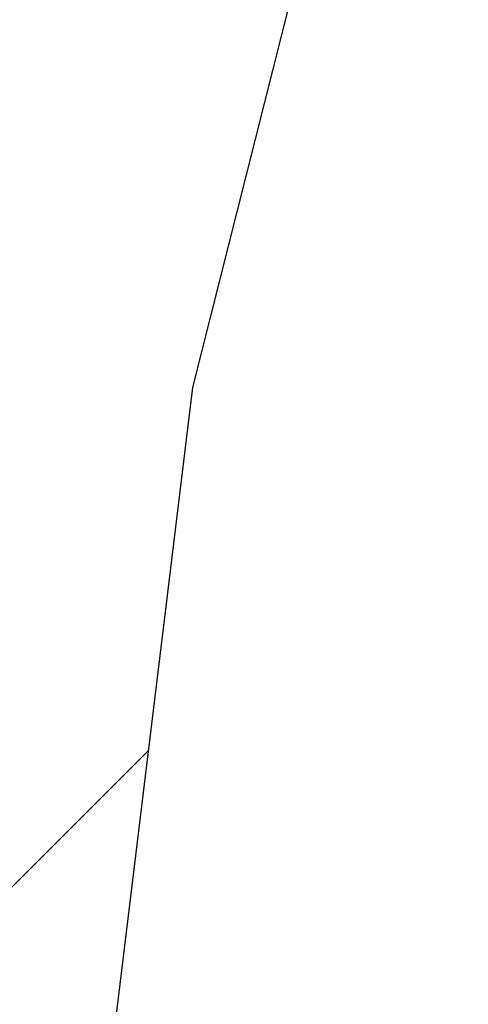
# Model space of a CAD drawing. Units: inches. Extents: x 3590 to 5167, y 65 to 1917.
# Tile 79 of 100: x 5049.155 to 5050.01, y 1787.154 to 1789.032. Entities that reach past the tile are written whole.
import ezdxf

# ---------------------------------------------------------------- set-up
doc = ezdxf.new("R2010")
doc.units = ezdxf.units.IN
for name, color, linetype, lineweight in [('A-ANNO-DIMS', 2, 'Continuous', 18), ('A-FLOR-PATT', 8, 'Continuous', 13), ('L-PLNT', 94, 'Continuous', 18)]:
    doc.layers.add(name, color=color, linetype=linetype, lineweight=lineweight)
doc.layers.add('DIENHOA', color=3, linetype='Continuous')
doc.styles.get("Standard").update_dxf_attribs({"font": 'arial.ttf'})
doc.dimstyles.new('ISO-25', dxfattribs={"dimtxt": 9, "dimasz": 2.5, "dimexe": 1.25, "dimexo": 0.625, "dimtad": 1, "dimdec": 1, "dimlunit": 3, "dimtxsty": 'Standard', "dimcen": 2.5, "dimadec": 0, "dimazin": 0, "dimtfac": 1, "dimtdec": 1, "dimtmove": 0, "dimatfit": 3, "dimfxl": 1, "dimarcsym": 0})

# ---------------------------------------------------------------- blocks, each defined once
blk = doc.blocks.new('Cay03_mb')
at = {"layer": 'DIENHOA'}
blk.add_lwpolyline([(-16.392, -26.735), (-38.342, 79.959), (-48.875, 178.33), (-48.703, 268.997), (-38.535, 352.583), (-19.079, 429.708), (8.954, 500.992), (44.855, 567.058), (87.915, 628.525)], dxfattribs=at)
blk = doc.blocks.new('*D322')
at = {"layer": 'A-ANNO-DIMS', "color": 0, "lineweight": -2, "transparency": 16777216}
for p, q in [((5035.7437, 1766.1842), (5035.7437, 1761.199)), ((5064.812, 1766.1842), (5064.812, 1761.199)), ((5038.2437, 1762.449), (5062.312, 1762.449)), ((5064.812, 1762.449), (5166.9911, 1762.449))]:
    blk.add_line(p, q, dxfattribs=at)
at = {"layer": 'A-ANNO-DIMS', "color": 0, "transparency": 16777216}
for points in [[(5038.2437, 1762.8657), (5038.2437, 1762.0323), (5035.7437, 1762.449)], [(5062.312, 1762.8657), (5062.312, 1762.0323), (5064.812, 1762.449)]]:
    blk.add_solid(points, dxfattribs=at)
at = {"layer": 'Defpoints', "color": 0, "transparency": 16777216}
for p in [(5035.7437, 1766.8092), (5064.812, 1766.8092), (5064.812, 1762.449)]:
    blk.add_point(p, dxfattribs=at)
at = {"layer": 'A-ANNO-DIMS', "color": 0, "transparency": 16777216, "insert": (5117.1516, 1767.6692), "char_height": 9, "attachment_point": 5}
blk.add_mtext('PLANT 2\'-5" TYP.', dxfattribs=at)

msp = doc.modelspace()

# ---------------------------------------------------------------- hatches: boundary and pattern name
at = {"layer": 'A-FLOR-PATT', "transparency": 33554687}
h = msp.add_hatch(dxfattribs=at)
h.set_pattern_fill('AR-HBONE', color=256, scale=0.2)
h.set_pattern_definition([(45, (-588.972, 0), (0, 28.73682), [60.96, -20.32]), (135, (-574.604, 14.368), (3e-15, 28.73682), [60.96, -20.32])])
h.paths.add_polyline_path([(5071.274, 1796.999), (4933.274, 1796.999), (4933.274, 1753.999), (4962.774, 1753.999, -0.414214), (4928.774, 1719.999), (4933.274, 1718.999), (4933.274, 1334.999), (5071.274, 1334.999)])
h.paths.add_polyline_path([(4951.78, 1521.0767), (4951.7151, 1521.0404), (4951.5634, 1520.8953)], flags=16)
h.paths.add_polyline_path([(4952.267, 1521.3764), (4952.1977, 1521.3711), (4952.1982, 1521.3556)], flags=0)
h.paths.add_polyline_path([(4967.0508, 1529.7283), (4965.2312, 1528.6944), (4963.4111, 1527.714), (4961.7565, 1526.8508), (4963.5889, 1527.4494), (4964.0356, 1527.478), (4962.9755, 1527.249), (4961.7602, 1526.852), (4959.7922, 1525.8341), (4958.005, 1524.8948), (4956.2403, 1523.9296), (4954.5039, 1522.9185), (4954.1294, 1522.6816), (4953.3605, 1521.9969), (4953.3656, 1521.9975), (4953.605, 1522.0637), (4955.1061, 1522.7608), (4956.9211, 1523.4341), (4958.6778, 1523.9151), (4960.3583, 1524.2004), (4961.9446, 1524.2861), (4964.1714, 1524.1085), (4965.9575, 1523.309), (4963.8627, 1522.9756), (4965.1874, 1522.499), (4963.3661, 1522.4971), (4961.5453, 1522.4868), (4959.7636, 1522.4608), (4958.3041, 1522.4188), (4957.9736, 1522.3883), (4956.3069, 1522.2324), (4954.7182, 1522.0714), (4953.2508, 1521.8992), (4953.5251, 1521.6228), (4954.3309, 1521.3788), (4956.2426, 1521.2299), (4958.0391, 1520.9295), (4959.6842, 1520.4834), (4961.1601, 1519.8957), (4963.107, 1518.8002), (4964.3929, 1517.3252), (4962.9731, 1517.726), (4964.5584, 1516.6606), (4965.4066, 1515.7078), (4963.5073, 1516.3218), (4961.68, 1517.0051), (4959.9348, 1517.7449), (4958.2821, 1518.5283), (4956.7322, 1519.3426), (4955.2953, 1520.1748), (4954.6715, 1520.5724), (4954.5128, 1520.6271), (4955.6585, 1519.3184), (4956.7026, 1517.9823), (4957.644, 1516.6466), (4958.4855, 1515.3344), (4959.55, 1513.524), (4960.4377, 1511.7694), (4958.8411, 1513.6196), (4957.4517, 1515.3249), (4955.8186, 1517.4586), (4956.6654, 1515.4476), (4957.1111, 1513.9229), (4957.4468, 1511.7143), (4957.0764, 1509.7929), (4956.5376, 1511.1103), (4955.9923, 1512.5689), (4955.4445, 1514.1251), (4954.8979, 1515.7352), (4954.3565, 1517.3555), (4953.8241, 1518.9425), (4953.3046, 1520.4525), (4953.0645, 1521.1156), (4952.9714, 1521.1461), (4952.9493, 1521.0865), (4952.7298, 1520.199), (4953.3698, 1518.0236), (4953.7571, 1516.3728), (4954.0512, 1514.7654), (4954.2645, 1513.2212), (4954.4712, 1511.1312), (4954.4971, 1510.4017), (4954.409, 1511.7601), (4954.2645, 1513.2212), (4954.0512, 1514.7654), (4953.7571, 1516.3728), (4953.3698, 1518.0236), (4952.8772, 1519.6981), (4952.7161, 1520.1412), (4952.533, 1519.0587), (4952.3743, 1517.7888), (4952.2192, 1516.3117), (4952.046, 1514.5999), (4951.8325, 1512.626), (4951.557, 1510.3626), (4951.2033, 1512.1682), (4950.8517, 1514.3393), (4950.9853, 1516.3759), (4951.6596, 1518.2862), (4952.5926, 1520.4808), (4952.3566, 1521.1299), (4951.855, 1520.3275), (4950.839, 1518.9083), (4949.7767, 1517.5866), (4948.9155, 1516.6173), (4948.111, 1515.2561), (4947.0891, 1513.5539), (4945.8894, 1511.6149), (4946.3259, 1513.4023), (4946.5624, 1514.2491), (4945.5277, 1513.3267), (4944.5811, 1512.5313), (4946.0177, 1514.5082), (4947.2044, 1516.0476), (4947.8933, 1517.3133), (4949.3069, 1518.7645), (4950.4142, 1519.7672), (4950.4513, 1519.8063), (4952.267, 1521.3764), (4951.6446, 1521.4932), (4950.4037, 1521.1795), (4948.0445, 1520.3587), (4946.1186, 1519.452), (4944.5718, 1518.4748), (4943.3496, 1517.4427), (4941.997, 1515.9197), (4941.6615, 1515.2748), (4942.8133, 1516.9897), (4944.5718, 1518.4748), (4946.1186, 1519.452), (4948.0445, 1520.3587), (4950.4037, 1521.1795), (4951.6446, 1521.4932), (4949.6468, 1521.8678), (4948.5998, 1521.7563), (4947.1263, 1521.5699), (4945.4202, 1521.3476), (4943.4497, 1521.1046), (4941.1832, 1520.856), (4942.8603, 1521.6126), (4943.8731, 1522.0301), (4942.9522, 1521.9093), (4941.4097, 1521.4851), (4939.5429, 1520.6702), (4938.9677, 1520.2255), (4940.7328, 1521.299), (4942.9522, 1521.9093), (4943.7018, 1522.0077), (4945.8942, 1522.7), (4947.5649, 1522.714), (4948.9209, 1522.5657), (4951.1314, 1522.1827), (4950.9706, 1522.2969), (4948.1292, 1523.0056), (4946.035, 1523.7067), (4944.2323, 1524.5214), (4942.7069, 1525.4611), (4941.4442, 1526.5371), (4940.4297, 1527.7606), (4939.6489, 1529.1431), (4941.4209, 1528.1223), (4943.1474, 1527.1325), (4944.8409, 1526.1746), (4946.5139, 1525.2496), (4948.1789, 1524.3586), (4948.3646, 1524.2634), (4946.4753, 1526.0446), (4945.1808, 1527.5404), (4944.1904, 1529.0334), (4943.4956, 1530.5398), (4943.2781, 1531.3597), (4942.4985, 1531.919), (4943.1135, 1531.7625), (4942.9593, 1533.6586), (4944.1395, 1531.9886), (4944.6117, 1531.3234), (4946.2016, 1530.4634), (4947.4857, 1529.5093), (4948.7903, 1528.2265), (4950.3675, 1526.2375), (4949.4855, 1528.1555), (4948.8513, 1530.1225), (4948.4905, 1532.0413), (4948.3811, 1533.9182), (4948.5006, 1535.7599), (4948.827, 1537.5728), (4949.418, 1535.5653), (4949.9568, 1533.5693), (4950.4641, 1531.5861), (4950.9606, 1529.6167), (4951.3911, 1527.9545), (4951.7235, 1530.6869), (4952.2011, 1532.5799), (4952.8891, 1534.3296), (4953.7703, 1535.9512), (4954.8273, 1537.46), (4954.5214, 1535.3897), (4954.2731, 1533.9368), (4955.58, 1535.6627), (4956.7476, 1536.7386), (4956.1585, 1534.7803), (4955.5892, 1532.8733), (4955.0434, 1531.0058), (4954.5249, 1529.1658), (4954.0377, 1527.3413), (4953.6383, 1525.733), (4953.6114, 1525.5856), (4953.3981, 1524.1657), (4953.3822, 1524.0089), (4954.0696, 1525.4756), (4954.9121, 1527.0217), (4956.1363, 1528.8935), (4957.8467, 1530.577), (4959.376, 1531.5401), (4958.256, 1530.104), (4957.1428, 1528.6629), (4956.0663, 1527.2431), (4955.0558, 1525.8705), (4954.141, 1524.5715), (4953.3516, 1523.372), (4953.3108, 1523.303), (4953.2725, 1522.9248), (4953.261, 1522.3821), (4954.1031, 1523.3727), (4954.63, 1524.2838), (4955.9615, 1526.3577), (4957.23, 1528.1297), (4958.4206, 1529.6086), (4960.0367, 1531.3679), (4961.3736, 1532.3752), (4962.1015, 1532.77), (4961.0699, 1531.0611), (4959.9873, 1529.4381), (4958.8685, 1527.908), (4958.1505, 1527.0074), (4959.8029, 1528.0031), (4961.5885, 1528.7926), (4963.3909, 1529.3278), (4965.2112, 1529.6321)], flags=16)
h.paths.add_polyline_path([(4962.9439, 1523.1819), (4961.1071, 1523.4219), (4960.3921, 1523.3616), (4962.3496, 1523.3306)], flags=0)
h.paths.add_polyline_path([(5049.5413, 1584.5509), (5049.4764, 1584.5146), (5049.3247, 1584.3695)], flags=16)
h.paths.add_polyline_path([(5050.0283, 1584.8506), (5049.959, 1584.8453), (5049.9595, 1584.8298)], flags=0)
h.paths.add_polyline_path([(5042.3331, 1581.949), (5043.8799, 1582.9262), (5045.8057, 1583.8329), (5048.165, 1584.6537), (5049.4058, 1584.9674), (5047.408, 1585.342), (5046.3611, 1585.2305), (5044.8876, 1585.0441), (5043.1814, 1584.8218), (5041.211, 1584.5788), (5038.9445, 1584.3301), (5040.6215, 1585.0868), (5041.6343, 1585.5043), (5040.7134, 1585.3835), (5039.1709, 1584.9593), (5037.3041, 1584.1444), (5036.729, 1583.6997), (5038.4941, 1584.7732), (5040.7134, 1585.3835), (5041.4631, 1585.4819), (5043.6555, 1586.1742), (5045.3261, 1586.1882), (5046.6821, 1586.0399), (5048.8927, 1585.6569), (5048.7319, 1585.7711), (5045.8905, 1586.4798), (5043.7962, 1587.1809), (5041.9936, 1587.9956), (5040.4682, 1588.9353), (5039.2055, 1590.0113), (5038.1909, 1591.2348), (5037.4102, 1592.6172), (5039.1822, 1591.5965), (5040.9087, 1590.6067), (5042.6022, 1589.6488), (5044.2752, 1588.7238), (5045.9402, 1587.8327), (5046.1258, 1587.7375), (5044.2366, 1589.5188), (5042.9421, 1591.0146), (5041.9517, 1592.5076), (5041.2569, 1594.014), (5041.0393, 1594.8339), (5040.2598, 1595.3932), (5040.8748, 1595.2367), (5040.7205, 1597.1328), (5041.9008, 1595.4628), (5042.373, 1594.7976), (5043.9629, 1593.9376), (5045.2469, 1592.9834), (5046.5515, 1591.7007), (5048.1288, 1589.7116), (5047.2467, 1591.6297), (5046.6125, 1593.5967), (5046.2518, 1595.5155), (5046.1423, 1597.3924), (5046.2619, 1599.2341), (5046.5883, 1601.047), (5047.1793, 1599.0394), (5047.7181, 1597.0435), (5048.2254, 1595.0603), (5048.7218, 1593.0909), (5049.1524, 1591.4287), (5049.4848, 1594.1611), (5049.9623, 1596.0541), (5050.6504, 1597.8038), (5051.5316, 1599.4254), (5052.5885, 1600.9341), (5052.2827, 1598.8638), (5052.0344, 1597.411), (5053.3413, 1599.1369), (5054.5088, 1600.2128), (5053.9198, 1598.2545), (5053.3504, 1596.3475), (5052.8046, 1594.48), (5052.2862, 1592.6399), (5051.799, 1590.8155), (5051.3996, 1589.2072), (5051.3727, 1589.0598), (5051.1593, 1587.6398), (5051.1435, 1587.4831), (5051.8308, 1588.9498), (5052.6734, 1590.4959), (5053.8975, 1592.3677), (5055.6079, 1594.0512), (5057.1373, 1595.0143), (5056.0172, 1593.5782), (5054.9041, 1592.1371), (5053.8275, 1590.7172), (5052.8171, 1589.3447), (5051.9023, 1588.0457), (5051.1129, 1586.8462), (5051.0721, 1586.7772), (5051.0338, 1586.399), (5051.0223, 1585.8563), (5051.8644, 1586.8469), (5052.3913, 1587.7579), (5053.7228, 1589.8318), (5054.9913, 1591.6039), (5056.1818, 1593.0828), (5057.798, 1594.8421), (5059.1349, 1595.8494), (5059.8628, 1596.2442), (5058.8312, 1594.5353), (5057.7486, 1592.9123), (5056.6298, 1591.3822), (5055.9117, 1590.4816), (5057.5642, 1591.4773), (5059.3498, 1592.2667), (5061.1521, 1592.802), (5062.9724, 1593.1062), (5064.812, 1593.2025), (5062.9925, 1592.1686), (5061.1724, 1591.1882), (5059.5178, 1590.325), (5061.3501, 1590.9236), (5061.7968, 1590.9522), (5060.7368, 1590.7232), (5059.5215, 1590.3262), (5057.5535, 1589.3082), (5055.7662, 1588.369), (5054.0016, 1587.4038), (5052.2652, 1586.3927), (5051.8907, 1586.1558), (5051.1218, 1585.4711), (5051.1268, 1585.4717), (5051.3663, 1585.5379), (5052.8673, 1586.235), (5054.6823, 1586.9082), (5056.4391, 1587.3893), (5058.1196, 1587.6745), (5059.7058, 1587.7602), (5061.9327, 1587.5827), (5063.7188, 1586.7832), (5061.624, 1586.4498), (5062.9487, 1585.9732), (5061.1274, 1585.9713), (5059.3065, 1585.961), (5057.5249, 1585.935), (5056.0654, 1585.893), (5055.7348, 1585.8625), (5054.0682, 1585.7066), (5052.4795, 1585.5456), (5051.012, 1585.3733), (5051.2864, 1585.097), (5052.0921, 1584.853), (5054.0039, 1584.7041), (5055.8004, 1584.4037), (5057.4455, 1583.9576), (5058.9213, 1583.3699), (5060.8683, 1582.2744), (5062.1541, 1580.7994), (5060.7343, 1581.2001), (5062.3197, 1580.1348), (5063.1679, 1579.182), (5061.2686, 1579.796), (5059.4412, 1580.4793), (5057.696, 1581.2191), (5056.0434, 1582.0025), (5054.4934, 1582.8168), (5053.0565, 1583.649), (5052.4328, 1584.0466), (5052.2741, 1584.1013), (5053.4197, 1582.7925), (5054.4639, 1581.4565), (5055.4053, 1580.1208), (5056.2467, 1578.8086), (5057.3112, 1576.9982), (5058.1989, 1575.2435), (5056.6023, 1577.0938), (5055.213, 1578.7991), (5053.5799, 1580.9327), (5054.4266, 1578.9218), (5054.8724, 1577.3971), (5055.2081, 1575.1885), (5054.8377, 1573.2671), (5054.2988, 1574.5845), (5053.7536, 1576.0431), (5053.2057, 1577.5993), (5052.6592, 1579.2094), (5052.1178, 1580.8297), (5051.5854, 1582.4167), (5051.0658, 1583.9267), (5050.8258, 1584.5898), (5050.7327, 1584.6203), (5050.7106, 1584.5606), (5050.4911, 1583.6732), (5051.1311, 1581.4978), (5051.5183, 1579.847), (5051.8125, 1578.2396), (5052.0257, 1576.6954), (5052.2325, 1574.6054), (5052.2584, 1573.8759), (5052.1703, 1575.2342), (5052.0257, 1576.6954), (5051.8125, 1578.2396), (5051.5183, 1579.847), (5051.1311, 1581.4978), (5050.6384, 1583.1723), (5050.4774, 1583.6154), (5050.2943, 1582.5329), (5050.1355, 1581.263), (5049.9805, 1579.7859), (5049.8072, 1578.074), (5049.5938, 1576.1002), (5049.3182, 1573.8368), (5048.9646, 1575.6424), (5048.6129, 1577.8135), (5048.7466, 1579.8501), (5049.4209, 1581.7604), (5050.3539, 1583.955), (5050.1179, 1584.6041), (5049.6163, 1583.8017), (5048.6003, 1582.3825), (5047.538, 1581.0608), (5046.6768, 1580.0915), (5045.8722, 1578.7303), (5044.8504, 1577.0281), (5043.6506, 1575.0891), (5044.0871, 1576.8765), (5044.3237, 1577.7233), (5043.289, 1576.8009), (5042.3423, 1576.0054), (5043.779, 1577.9824), (5044.9657, 1579.5218), (5045.6546, 1580.7875), (5047.0681, 1582.2386), (5048.1754, 1583.2413), (5048.2126, 1583.2805), (5050.0283, 1584.8506), (5049.4058, 1584.9674), (5048.165, 1584.6537), (5045.8057, 1583.8329), (5043.8799, 1582.9262), (5042.3331, 1581.949), (5041.1109, 1580.9168), (5039.7582, 1579.3939), (5039.4227, 1578.7489), (5040.5746, 1580.4639)], flags=16)
h.paths.add_polyline_path([(4954.7987, 1533.1203), (4954.2625, 1532.0793), (4953.8311, 1530.9346), (4953.5047, 1529.636), (4953.2834, 1528.1333), (4953.1672, 1526.3764), (4953.1563, 1524.315), (4953.2767, 1521.2363), (4952.8017, 1521.8418), (4951.557, 1521.9979), (4950.9758, 1521.9613), (4952.6606, 1521.941), (4952.8017, 1521.8418), (4953.1525, 1523.5926), (4953.1672, 1526.3764), (4953.2834, 1528.1333), (4953.6093, 1530.346), (4954.4556, 1532.5917)], flags=0)
h.paths.add_polyline_path([(5050.5629, 1585.316), (5049.3182, 1585.4721), (5048.737, 1585.4355), (5050.4219, 1585.4152), (5050.5629, 1585.316), (5050.9138, 1587.0668), (5050.9285, 1589.8506), (5051.0446, 1591.6075), (5051.3706, 1593.8202), (5052.2168, 1596.0659), (5052.56, 1596.5945), (5052.0238, 1595.5535), (5051.5924, 1594.4088), (5051.266, 1593.1102), (5051.0446, 1591.6075), (5050.9285, 1589.8506), (5050.9176, 1587.7892), (5051.038, 1584.7105)], flags=0)
h.paths.add_polyline_path([(5058.1533, 1586.8358), (5060.1109, 1586.8048), (5060.7051, 1586.6561), (5058.8684, 1586.8961)], flags=0)
h.paths.add_polyline_path([(5049.5413, 1430.9361), (5049.4764, 1430.8998), (5049.3247, 1430.7547)], flags=16)
h.paths.add_polyline_path([(5050.0283, 1431.2359), (5049.959, 1431.2305), (5049.9595, 1431.215)], flags=0)
h.paths.add_polyline_path([(5046.5883, 1447.4322), (5047.1793, 1445.4247), (5047.7181, 1443.4287), (5048.2254, 1441.4455), (5048.7218, 1439.4761), (5049.1524, 1437.8139), (5049.4848, 1440.5463), (5049.9623, 1442.4393), (5050.6504, 1444.189), (5051.5316, 1445.8106), (5052.5885, 1447.3194), (5052.2827, 1445.2491), (5052.0344, 1443.7962), (5053.3413, 1445.5221), (5054.5088, 1446.598), (5053.9198, 1444.6397), (5053.3504, 1442.7327), (5052.8046, 1440.8652), (5052.2862, 1439.0252), (5051.799, 1437.2007), (5051.3996, 1435.5924), (5051.3727, 1435.445), (5051.1593, 1434.0251), (5051.1435, 1433.8683), (5051.8308, 1435.335), (5052.6734, 1436.8811), (5053.8975, 1438.7529), (5055.6079, 1440.4364), (5057.1373, 1441.3995), (5056.0172, 1439.9634), (5054.9041, 1438.5223), (5053.8275, 1437.1025), (5052.8171, 1435.7299), (5051.9023, 1434.4309), (5051.1129, 1433.2314), (5051.0721, 1433.1624), (5051.0338, 1432.7842), (5051.0223, 1432.2415), (5051.8644, 1433.2321), (5052.3913, 1434.1432), (5053.7228, 1436.2171), (5054.9913, 1437.9891), (5056.1818, 1439.468), (5057.798, 1441.2273), (5059.1349, 1442.2346), (5059.8628, 1442.6294), (5058.8312, 1440.9205), (5057.7486, 1439.2975), (5056.6298, 1437.7674), (5055.9117, 1436.8668), (5057.5642, 1437.8625), (5059.3498, 1438.652), (5061.1521, 1439.1872), (5062.9724, 1439.4915), (5064.812, 1439.5877), (5062.9925, 1438.5538), (5061.1724, 1437.5734), (5059.5178, 1436.7102), (5061.3501, 1437.3088), (5061.7968, 1437.3374), (5060.7368, 1437.1084), (5059.5215, 1436.7114), (5057.5535, 1435.6935), (5055.7662, 1434.7542), (5054.0016, 1433.789), (5052.2652, 1432.7779), (5051.8907, 1432.541), (5051.1218, 1431.8563), (5051.1268, 1431.8569), (5051.3663, 1431.9231), (5052.8673, 1432.6202), (5054.6823, 1433.2935), (5056.4391, 1433.7745), (5058.1196, 1434.0598), (5059.7058, 1434.1455), (5061.9327, 1433.9679), (5063.7188, 1433.1684), (5061.624, 1432.8351), (5062.9487, 1432.3584), (5061.1274, 1432.3566), (5059.3065, 1432.3462), (5057.5249, 1432.3202), (5056.0654, 1432.2782), (5055.7348, 1432.2477), (5054.0682, 1432.0918), (5052.4795, 1431.9308), (5051.012, 1431.7586), (5051.2864, 1431.4822), (5052.0921, 1431.2382), (5054.0039, 1431.0893), (5055.8004, 1430.7889), (5057.4455, 1430.3428), (5058.9213, 1429.7551), (5060.8683, 1428.6596), (5062.1541, 1427.1846), (5060.7343, 1427.5854), (5062.3197, 1426.52), (5063.1679, 1425.5672), (5061.2686, 1426.1812), (5059.4412, 1426.8645), (5057.696, 1427.6043), (5056.0434, 1428.3877), (5054.4934, 1429.202), (5053.0565, 1430.0342), (5052.4328, 1430.4318), (5052.2741, 1430.4865), (5053.4197, 1429.1778), (5054.4639, 1427.8417), (5055.4053, 1426.506), (5056.2467, 1425.1938), (5057.3112, 1423.3834), (5058.1989, 1421.6288), (5056.6023, 1423.479), (5055.213, 1425.1843), (5053.5799, 1427.318), (5054.4266, 1425.307), (5054.8724, 1423.7823), (5055.2081, 1421.5737), (5054.8377, 1419.6523), (5054.2988, 1420.9697), (5053.7536, 1422.4283), (5053.2057, 1423.9845), (5052.6592, 1425.5946), (5052.1178, 1427.2149), (5051.5854, 1428.8019), (5051.0658, 1430.3119), (5050.8258, 1430.975), (5050.7327, 1431.0055), (5050.7106, 1430.9459), (5050.4911, 1430.0585), (5051.1311, 1427.883), (5051.5183, 1426.2322), (5051.8125, 1424.6248), (5052.0257, 1423.0806), (5052.2325, 1420.9906), (5052.2584, 1420.2611), (5052.1703, 1421.6195), (5052.0257, 1423.0806), (5051.8125, 1424.6248), (5051.5183, 1426.2322), (5051.1311, 1427.883), (5050.6384, 1429.5575), (5050.4774, 1430.0006), (5050.2943, 1428.9181), (5050.1355, 1427.6482), (5049.9805, 1426.1711), (5049.8072, 1424.4593), (5049.5938, 1422.4854), (5049.3182, 1420.222), (5048.9646, 1422.0276), (5048.6129, 1424.1987), (5048.7466, 1426.2353), (5049.4209, 1428.1457), (5050.3539, 1430.3403), (5050.1179, 1430.9893), (5049.6163, 1430.1869), (5048.6003, 1428.7677), (5047.538, 1427.446), (5046.6768, 1426.4767), (5045.8722, 1425.1155), (5044.8504, 1423.4133), (5043.6506, 1421.4744), (5044.0871, 1423.2617), (5044.3237, 1424.1085), (5043.289, 1423.1861), (5042.3423, 1422.3907), (5043.779, 1424.3677), (5044.9657, 1425.907), (5045.6546, 1427.1727), (5047.0681, 1428.6239), (5048.1754, 1429.6266), (5048.2126, 1429.6657), (5050.0283, 1431.2359), (5049.4058, 1431.3526), (5048.165, 1431.0389), (5045.8057, 1430.2181), (5043.8799, 1429.3114), (5042.3331, 1428.3342), (5041.1109, 1427.3021), (5039.7582, 1425.7791), (5039.4227, 1425.1342), (5040.5746, 1426.8491), (5042.3331, 1428.3342), (5043.8799, 1429.3114), (5045.8057, 1430.2181), (5048.165, 1431.0389), (5049.4058, 1431.3526), (5047.408, 1431.7272), (5046.3611, 1431.6157), (5044.8876, 1431.4293), (5043.1814, 1431.207), (5041.211, 1430.964), (5038.9445, 1430.7154), (5040.6215, 1431.4721), (5041.6343, 1431.8895), (5040.7134, 1431.7687), (5039.1709, 1431.3445), (5037.3041, 1430.5296), (5036.729, 1430.0849), (5038.4941, 1431.1584), (5040.7134, 1431.7687), (5041.4631, 1431.8671), (5043.6555, 1432.5594), (5045.3261, 1432.5734), (5046.6821, 1432.4251), (5048.8927, 1432.0421), (5048.7319, 1432.1563), (5045.8905, 1432.865), (5043.7962, 1433.5661), (5041.9936, 1434.3808), (5040.4682, 1435.3205), (5039.2055, 1436.3965), (5038.1909, 1437.62), (5037.4102, 1439.0025), (5039.1822, 1437.9817), (5040.9087, 1436.9919), (5042.6022, 1436.034), (5044.2752, 1435.109), (5045.9402, 1434.218), (5046.1258, 1434.1228), (5044.2366, 1435.904), (5042.9421, 1437.3998), (5041.9517, 1438.8928), (5041.2569, 1440.3993), (5041.0393, 1441.2191), (5040.2598, 1441.7784), (5040.8748, 1441.6219), (5040.7205, 1443.518), (5041.9008, 1441.848), (5042.373, 1441.1828), (5043.9629, 1440.3228), (5045.2469, 1439.3687), (5046.5515, 1438.0859), (5048.1288, 1436.0969), (5047.2467, 1438.0149), (5046.6125, 1439.9819), (5046.2518, 1441.9007), (5046.1423, 1443.7776), (5046.2619, 1445.6193)], flags=16)
h.paths.add_polyline_path([(5052.3818, 1444.255), (5051.6226, 1442.7799), (5052.0238, 1441.9388), (5052.56, 1442.9797)], flags=0)
h.paths.add_polyline_path([(5050.5629, 1431.7012), (5049.3182, 1431.8573), (5048.737, 1431.8207), (5050.4219, 1431.8004)], flags=0)
h.paths.add_polyline_path([(5058.1533, 1433.221), (5060.1109, 1433.19), (5060.7051, 1433.0413), (5058.8684, 1433.2813)], flags=0)
h.paths.add_polyline_path([(5049.5413, 1352.2853), (5049.4764, 1352.249), (5049.3247, 1352.104)], flags=16)
h.paths.add_polyline_path([(5050.0283, 1352.5851), (5049.959, 1352.5797), (5049.9595, 1352.5642)], flags=0)
h.paths.add_polyline_path([(5046.5883, 1368.7815), (5047.1793, 1366.7739), (5047.7181, 1364.778), (5048.2254, 1362.7947), (5048.7218, 1360.8253), (5049.1524, 1359.1631), (5049.4848, 1361.8955), (5049.9623, 1363.7886), (5050.6504, 1365.5383), (5051.5316, 1367.1599), (5052.5885, 1368.6686), (5052.2827, 1366.5983), (5052.0344, 1365.1455), (5053.3413, 1366.8713), (5054.5088, 1367.9472), (5053.9198, 1365.9889), (5053.3504, 1364.082), (5052.8046, 1362.2144), (5052.2862, 1360.3744), (5051.799, 1358.5499), (5051.3996, 1356.9416), (5051.3727, 1356.7943), (5051.1593, 1355.3743), (5051.1435, 1355.2175), (5051.8308, 1356.6843), (5052.6734, 1358.2304), (5053.8975, 1360.1022), (5055.6079, 1361.7857), (5057.1373, 1362.7488), (5056.0172, 1361.3126), (5054.9041, 1359.8716), (5053.8275, 1358.4517), (5052.8171, 1357.0792), (5051.9023, 1355.7801), (5051.1129, 1354.5807), (5051.0721, 1354.5116), (5051.0338, 1354.1334), (5051.0223, 1353.5908), (5051.8644, 1354.5814), (5052.3913, 1355.4924), (5053.7228, 1357.5663), (5054.9913, 1359.3383), (5056.1818, 1360.8173), (5057.798, 1362.5766), (5059.1349, 1363.5838), (5059.8628, 1363.9786), (5058.8312, 1362.2698), (5057.7486, 1360.6468), (5056.6298, 1359.1167), (5055.9117, 1358.2161), (5057.5642, 1359.2118), (5059.3498, 1360.0012), (5061.1521, 1360.5365), (5062.9724, 1360.8407), (5064.812, 1360.937), (5062.9925, 1359.9031), (5061.1724, 1358.9227), (5059.5178, 1358.0595), (5061.3501, 1358.658), (5061.7968, 1358.6867), (5060.7368, 1358.4577), (5059.5215, 1358.0607), (5057.5535, 1357.0427), (5055.7662, 1356.1035), (5054.0016, 1355.1382), (5052.2652, 1354.1272), (5051.8907, 1353.8903), (5051.1218, 1353.2055), (5051.1268, 1353.2062), (5051.3663, 1353.2723), (5052.8673, 1353.9695), (5054.6823, 1354.6427), (5056.4391, 1355.1238), (5058.1196, 1355.409), (5059.7058, 1355.4947), (5061.9327, 1355.3171), (5063.7188, 1354.5177), (5061.624, 1354.1843), (5062.9487, 1353.7076), (5061.1274, 1353.7058), (5059.3065, 1353.6955), (5057.5249, 1353.6694), (5056.0654, 1353.6274), (5055.7348, 1353.5969), (5054.0682, 1353.441), (5052.4795, 1353.2801), (5051.012, 1353.1078), (5051.2864, 1352.8314), (5052.0921, 1352.5875), (5054.0039, 1352.4385), (5055.8004, 1352.1382), (5057.4455, 1351.692), (5058.9213, 1351.1043), (5060.8683, 1350.0089), (5062.1541, 1348.5338), (5060.7343, 1348.9346), (5062.3197, 1347.8692), (5063.1679, 1346.9164), (5061.2686, 1347.5304), (5059.4412, 1348.2137), (5057.696, 1348.9535), (5056.0434, 1349.737), (5054.4934, 1350.5512), (5053.0565, 1351.3834), (5052.4328, 1351.781), (5052.2741, 1351.8357), (5053.4197, 1350.527), (5054.4639, 1349.191), (5055.4053, 1347.8553), (5056.2467, 1346.543), (5057.3112, 1344.7326), (5058.1989, 1342.978), (5056.6023, 1344.8282), (5055.213, 1346.5335), (5053.5799, 1348.6672), (5054.4266, 1346.6563), (5054.8724, 1345.1316), (5055.2081, 1342.923), (5054.8377, 1341.0015), (5054.2988, 1342.3189), (5053.7536, 1343.7776), (5053.2057, 1345.3337), (5052.6592, 1346.9438), (5052.1178, 1348.5642), (5051.5854, 1350.1512), (5051.0658, 1351.6611), (5050.8258, 1352.3243), (5050.7327, 1352.3547), (5050.7106, 1352.2951), (5050.4911, 1351.4077), (5051.1311, 1349.2323), (5051.5183, 1347.5814), (5051.8125, 1345.974), (5052.0257, 1344.4298), (5052.2325, 1342.3399), (5052.2584, 1341.6104), (5052.1703, 1342.9687), (5052.0257, 1344.4298), (5051.8125, 1345.974), (5051.5183, 1347.5814), (5051.1311, 1349.2323), (5050.6384, 1350.9068), (5050.4774, 1351.3498), (5050.2943, 1350.2674), (5050.1355, 1348.9975), (5049.9805, 1347.5203), (5049.8072, 1345.8085), (5049.5938, 1343.8346), (5049.3182, 1341.5712), (5048.9646, 1343.3768), (5048.6129, 1345.548), (5048.7466, 1347.5846), (5049.4209, 1349.4949), (5050.3539, 1351.6895), (5050.1179, 1352.3385), (5049.6163, 1351.5362), (5048.6003, 1350.1169), (5047.538, 1348.7952), (5046.6768, 1347.826), (5045.8722, 1346.4647), (5044.8504, 1344.7625), (5043.6506, 1342.8236), (5044.0871, 1344.611), (5044.3237, 1345.4578), (5043.289, 1344.5353), (5042.3423, 1343.7399), (5043.779, 1345.7169), (5044.9657, 1347.2563), (5045.6546, 1348.522), (5047.0681, 1349.9731), (5048.1754, 1350.9758), (5048.2126, 1351.0149), (5050.0283, 1352.5851), (5049.4058, 1352.7018), (5048.165, 1352.3882), (5045.8057, 1351.5673), (5043.8799, 1350.6606), (5042.3331, 1349.6835), (5041.1109, 1348.6513), (5039.7582, 1347.1283), (5039.4227, 1346.4834), (5040.5746, 1348.1984), (5042.3331, 1349.6835), (5043.8799, 1350.6606), (5045.8057, 1351.5673), (5048.165, 1352.3882), (5049.4058, 1352.7018), (5047.408, 1353.0765), (5046.3611, 1352.965), (5044.8876, 1352.7785), (5043.1814, 1352.5563), (5041.211, 1352.3133), (5038.9445, 1352.0646), (5040.6215, 1352.8213), (5041.6343, 1353.2388), (5040.7134, 1353.1179), (5039.1709, 1352.6938), (5037.3041, 1351.8788), (5036.729, 1351.4341), (5038.4941, 1352.5076), (5040.7134, 1353.1179), (5041.4631, 1353.2163), (5043.6555, 1353.9086), (5045.3261, 1353.9226), (5046.6821, 1353.7744), (5048.8927, 1353.3914), (5048.7319, 1353.5055), (5045.8905, 1354.2143), (5043.7962, 1354.9153), (5041.9936, 1355.7301), (5040.4682, 1356.6698), (5039.2055, 1357.7457), (5038.1909, 1358.9693), (5037.4102, 1360.3517), (5039.1822, 1359.331), (5040.9087, 1358.3411), (5042.6022, 1357.3832), (5044.2752, 1356.4582), (5045.9402, 1355.5672), (5046.1258, 1355.472), (5044.2366, 1357.2532), (5042.9421, 1358.7491), (5041.9517, 1360.242), (5041.2569, 1361.7485), (5041.0393, 1362.5683), (5040.2598, 1363.1277), (5040.8748, 1362.9711), (5040.7205, 1364.8672), (5041.9008, 1363.1972), (5042.373, 1362.532), (5043.9629, 1361.6721), (5045.2469, 1360.7179), (5046.5515, 1359.4351), (5048.1288, 1357.4461), (5047.2467, 1359.3641), (5046.6125, 1361.3312), (5046.2518, 1363.2499), (5046.1423, 1365.1269), (5046.2619, 1366.9685)], flags=16)
h.paths.add_polyline_path([(5052.3818, 1365.6042), (5051.6226, 1364.1291), (5052.0238, 1363.288), (5052.56, 1364.3289)], flags=0)
h.paths.add_polyline_path([(4951.78, 1698.0408), (4951.7151, 1698.0045), (4951.5634, 1697.8594)], flags=16)
h.paths.add_polyline_path([(4952.267, 1698.3406), (4952.1977, 1698.3352), (4952.1982, 1698.3197)], flags=0)
h.paths.add_polyline_path([(4957.0764, 1686.757), (4956.5376, 1688.0744), (4955.9923, 1689.533), (4955.4445, 1691.0892), (4954.8979, 1692.6993), (4954.3565, 1694.3196), (4953.8241, 1695.9066), (4953.3046, 1697.4166), (4953.0645, 1698.0797), (4952.9714, 1698.1102), (4952.9493, 1698.0506), (4952.7298, 1697.1632), (4953.3698, 1694.9877), (4953.7571, 1693.3369), (4954.0512, 1691.7295), (4954.2645, 1690.1853), (4954.4712, 1688.0953), (4954.4971, 1687.3658), (4954.409, 1688.7242), (4954.2645, 1690.1853), (4954.0512, 1691.7295), (4953.7571, 1693.3369), (4953.3698, 1694.9877), (4952.8772, 1696.6622), (4952.7161, 1697.1053), (4952.533, 1696.0228), (4952.3743, 1694.7529), (4952.2192, 1693.2758), (4952.046, 1691.564), (4951.8325, 1689.5901), (4951.557, 1687.3267), (4951.2033, 1689.1323), (4950.8517, 1691.3034), (4950.9853, 1693.34), (4951.6596, 1695.2504), (4952.5926, 1697.445), (4952.3566, 1698.094), (4951.855, 1697.2916), (4950.839, 1695.8724), (4949.7767, 1694.5507), (4948.9155, 1693.5814), (4948.111, 1692.2202), (4947.0891, 1690.518), (4945.8894, 1688.5791), (4946.3259, 1690.3664), (4946.5624, 1691.2132), (4945.5277, 1690.2908), (4944.5811, 1689.4954), (4946.0177, 1691.4724), (4947.2044, 1693.0117), (4947.8933, 1694.2774), (4949.3069, 1695.7286), (4950.4142, 1696.7313), (4950.4513, 1696.7704), (4952.267, 1698.3406), (4951.6446, 1698.4573), (4950.4037, 1698.1436), (4948.0445, 1697.3228), (4946.1186, 1696.4161), (4944.5718, 1695.4389), (4943.3496, 1694.4068), (4941.997, 1692.8838), (4941.6615, 1692.2389), (4942.8133, 1693.9538), (4944.5718, 1695.4389), (4946.1186, 1696.4161), (4948.0445, 1697.3228), (4950.4037, 1698.1436), (4951.6446, 1698.4573), (4949.6468, 1698.8319), (4948.5998, 1698.7204), (4947.1263, 1698.534), (4945.4202, 1698.3117), (4943.4497, 1698.0687), (4941.1832, 1697.8201), (4942.8603, 1698.5768), (4943.8731, 1698.9942), (4942.9522, 1698.8734), (4941.4097, 1698.4492), (4939.5429, 1697.6343), (4938.9677, 1697.1896), (4940.7328, 1698.2631), (4942.9522, 1698.8734), (4943.7018, 1698.9718), (4945.8942, 1699.6641), (4947.5649, 1699.6781), (4948.9209, 1699.5298), (4951.1314, 1699.1468), (4950.9706, 1699.261), (4948.1292, 1699.9697), (4946.035, 1700.6708), (4944.2323, 1701.4855), (4942.7069, 1702.4252), (4941.4442, 1703.5012), (4940.4297, 1704.7247), (4939.6489, 1706.1072), (4941.4209, 1705.0864), (4943.1474, 1704.0966), (4944.8409, 1703.1387), (4946.5139, 1702.2137), (4948.1789, 1701.3227), (4948.3646, 1701.2275), (4946.4753, 1703.0087), (4945.1808, 1704.5045), (4944.1904, 1705.9975), (4943.4956, 1707.504), (4943.2781, 1708.3238), (4942.4985, 1708.8831), (4943.1135, 1708.7266), (4942.9593, 1710.6227), (4944.1395, 1708.9527), (4944.6117, 1708.2875), (4946.2016, 1707.4275), (4947.4857, 1706.4734), (4948.7903, 1705.1906), (4950.3675, 1703.2016), (4949.4855, 1705.1196), (4948.8513, 1707.0866), (4948.4905, 1709.0054), (4948.3811, 1710.8823), (4948.5006, 1712.724), (4948.827, 1714.5369), (4949.418, 1712.5294), (4949.9568, 1710.5334), (4950.4641, 1708.5502), (4950.9606, 1706.5808), (4951.3911, 1704.9186), (4951.7235, 1707.651), (4952.2011, 1709.544), (4952.8891, 1711.2937), (4953.7703, 1712.9153), (4954.8273, 1714.4241), (4954.5214, 1712.3538), (4954.2731, 1710.9009), (4955.58, 1712.6268), (4956.7476, 1713.7027), (4956.1585, 1711.7444), (4955.5892, 1709.8374), (4955.0434, 1707.9699), (4954.5249, 1706.1299), (4954.0377, 1704.3054), (4953.6383, 1702.6971), (4953.6114, 1702.5497), (4953.3981, 1701.1298), (4953.3822, 1700.973), (4954.0696, 1702.4397), (4954.9121, 1703.9858), (4956.1363, 1705.8576), (4957.8467, 1707.5411), (4959.376, 1708.5042), (4958.256, 1707.0681), (4957.1428, 1705.627), (4956.0663, 1704.2072), (4955.0558, 1702.8346), (4954.141, 1701.5356), (4953.3516, 1700.3361), (4953.3108, 1700.2671), (4953.2725, 1699.8889), (4953.261, 1699.3462), (4954.1031, 1700.3368), (4954.63, 1701.2479), (4955.9615, 1703.3218), (4957.23, 1705.0938), (4958.4206, 1706.5727), (4960.0367, 1708.332), (4961.3736, 1709.3393), (4962.1015, 1709.7341), (4961.0699, 1708.0252), (4959.9873, 1706.4022), (4958.8685, 1704.8721), (4958.1505, 1703.9715), (4959.8029, 1704.9672), (4961.5885, 1705.7567), (4963.3909, 1706.2919), (4965.2112, 1706.5962), (4967.0508, 1706.6924), (4965.2312, 1705.6585), (4963.4111, 1704.6781), (4961.7565, 1703.8149), (4963.5889, 1704.4135), (4964.0356, 1704.4421), (4962.9755, 1704.2131), (4961.7602, 1703.8161), (4959.7922, 1702.7982), (4958.005, 1701.8589), (4956.2403, 1700.8937), (4954.5039, 1699.8826), (4954.1294, 1699.6457), (4953.3605, 1698.961), (4953.3656, 1698.9616), (4953.605, 1699.0278), (4955.1061, 1699.7249), (4956.9211, 1700.3982), (4958.6778, 1700.8792), (4960.3583, 1701.1645), (4961.9446, 1701.2502), (4964.1714, 1701.0726), (4965.9575, 1700.2731), (4963.8627, 1699.9398), (4965.1874, 1699.4631), (4963.3661, 1699.4613), (4961.5453, 1699.4509), (4959.7636, 1699.4249), (4958.3041, 1699.3829), (4957.9736, 1699.3524), (4956.3069, 1699.1965), (4954.7182, 1699.0355), (4953.2508, 1698.8633), (4953.5251, 1698.5869), (4954.3309, 1698.3429), (4956.2426, 1698.194), (4958.0391, 1697.8936), (4959.6842, 1697.4475), (4961.1601, 1696.8598), (4963.107, 1695.7643), (4964.3929, 1694.2893), (4962.9731, 1694.6901), (4964.5584, 1693.6247), (4965.4066, 1692.6719), (4963.5073, 1693.2859), (4961.68, 1693.9692), (4959.9348, 1694.709), (4958.2821, 1695.4924), (4956.7322, 1696.3067), (4955.2953, 1697.1389), (4954.6715, 1697.5365), (4954.5128, 1697.5912), (4955.6585, 1696.2825), (4956.7026, 1694.9464), (4957.644, 1693.6107), (4958.4855, 1692.2985), (4959.55, 1690.4881), (4960.4377, 1688.7335), (4958.8411, 1690.5837), (4957.4517, 1692.289), (4955.8186, 1694.4227), (4956.6654, 1692.4117), (4957.1111, 1690.887), (4957.4468, 1688.6784)], flags=16)
h.paths.add_polyline_path([(5050.5629, 1353.0504), (5049.3182, 1353.2065), (5048.737, 1353.1699), (5050.4219, 1353.1496)], flags=0)
h.paths.add_polyline_path([(4951.78, 1351.4861), (4951.7151, 1351.4498), (4951.5634, 1351.3047)], flags=16)
h.paths.add_polyline_path([(4952.267, 1351.7858), (4952.1977, 1351.7805), (4952.1982, 1351.765)], flags=0)
h.paths.add_polyline_path([(4954.8273, 1367.8693), (4954.5214, 1365.799), (4954.2731, 1364.3462), (4955.58, 1366.0721), (4956.7476, 1367.148), (4956.1585, 1365.1897), (4955.5892, 1363.2827), (4955.0434, 1361.4152), (4954.5249, 1359.5752), (4954.0377, 1357.7507), (4953.6383, 1356.1424), (4953.6114, 1355.995), (4953.3981, 1354.575), (4953.3822, 1354.4183), (4954.0696, 1355.885), (4954.9121, 1357.4311), (4956.1363, 1359.3029), (4957.8467, 1360.9864), (4959.376, 1361.9495), (4958.256, 1360.5134), (4957.1428, 1359.0723), (4956.0663, 1357.6524), (4955.0558, 1356.2799), (4954.141, 1354.9809), (4953.3516, 1353.7814), (4953.3108, 1353.7124), (4953.2725, 1353.3342), (4953.261, 1352.7915), (4954.1031, 1353.7821), (4954.63, 1354.6931), (4955.9615, 1356.7671), (4957.23, 1358.5391), (4958.4206, 1360.018), (4960.0367, 1361.7773), (4961.3736, 1362.7846), (4962.1015, 1363.1794), (4961.0699, 1361.4705), (4959.9873, 1359.8475), (4958.8685, 1358.3174), (4958.1505, 1357.4168), (4959.8029, 1358.4125), (4961.5885, 1359.202), (4963.3909, 1359.7372), (4965.2112, 1360.0414), (4967.0508, 1360.1377), (4965.2312, 1359.1038), (4963.4111, 1358.1234), (4961.7565, 1357.2602), (4963.5889, 1357.8588), (4964.0356, 1357.8874), (4962.9755, 1357.6584), (4961.7602, 1357.2614), (4959.7922, 1356.2435), (4958.005, 1355.3042), (4956.2403, 1354.339), (4954.5039, 1353.3279), (4954.1294, 1353.091), (4953.3605, 1352.4063), (4953.3656, 1352.4069), (4953.605, 1352.4731), (4955.1061, 1353.1702), (4956.9211, 1353.8434), (4958.6778, 1354.3245), (4960.3583, 1354.6098), (4961.9446, 1354.6954), (4964.1714, 1354.5179), (4965.9575, 1353.7184), (4963.8627, 1353.385), (4965.1874, 1352.9084), (4963.3661, 1352.9065), (4961.5453, 1352.8962), (4959.7636, 1352.8702), (4958.3041, 1352.8282), (4957.9736, 1352.7977), (4956.3069, 1352.6418), (4954.7182, 1352.4808), (4953.2508, 1352.3085), (4953.5251, 1352.0322), (4954.3309, 1351.7882), (4956.2426, 1351.6393), (4958.0391, 1351.3389), (4959.6842, 1350.8928), (4961.1601, 1350.3051), (4963.107, 1349.2096), (4964.3929, 1347.7346), (4962.9731, 1348.1354), (4964.5584, 1347.07), (4965.4066, 1346.1172), (4963.5073, 1346.7312), (4961.68, 1347.4145), (4959.9348, 1348.1543), (4958.2821, 1348.9377), (4956.7322, 1349.752), (4955.2953, 1350.5842), (4954.6715, 1350.9818), (4954.5128, 1351.0365), (4955.6585, 1349.7278), (4956.7026, 1348.3917), (4957.644, 1347.056), (4958.4855, 1345.7438), (4959.55, 1343.9334), (4960.4377, 1342.1788), (4958.8411, 1344.029), (4957.4517, 1345.7343), (4955.8186, 1347.8679), (4956.6654, 1345.857), (4957.1111, 1344.3323), (4957.4468, 1342.1237), (4957.0764, 1340.2023), (4956.5376, 1341.5197), (4955.9923, 1342.9783), (4955.4445, 1344.5345), (4954.8979, 1346.1446), (4954.3565, 1347.7649), (4953.8241, 1349.3519), (4953.3046, 1350.8619), (4953.0645, 1351.525), (4952.9714, 1351.5555), (4952.9493, 1351.4959), (4952.7298, 1350.6084), (4953.3698, 1348.433), (4953.7571, 1346.7822), (4954.0512, 1345.1748), (4954.2645, 1343.6306), (4954.4712, 1341.5406), (4954.4971, 1340.8111), (4954.409, 1342.1695), (4954.2645, 1343.6306), (4954.0512, 1345.1748), (4953.7571, 1346.7822), (4953.3698, 1348.433), (4952.8772, 1350.1075), (4952.7161, 1350.5506), (4952.533, 1349.4681), (4952.3743, 1348.1982), (4952.2192, 1346.7211), (4952.046, 1345.0093), (4951.8325, 1343.0354), (4951.557, 1340.772), (4951.2033, 1342.5776), (4950.8517, 1344.7487), (4950.9853, 1346.7853), (4951.6596, 1348.6956), (4952.5926, 1350.8902), (4952.3566, 1351.5393), (4951.855, 1350.7369), (4950.839, 1349.3177), (4949.7767, 1347.996), (4948.9155, 1347.0267), (4948.111, 1345.6655), (4947.0891, 1343.9633), (4945.8894, 1342.0243), (4946.3259, 1343.8117), (4946.5624, 1344.6585), (4945.5277, 1343.7361), (4944.5811, 1342.9407), (4946.0177, 1344.9176), (4947.2044, 1346.457), (4947.8933, 1347.7227), (4949.3069, 1349.1739), (4950.4142, 1350.1766), (4950.4513, 1350.2157), (4952.267, 1351.7858), (4951.6446, 1351.9026), (4950.4037, 1351.5889), (4948.0445, 1350.7681), (4946.1186, 1349.8614), (4944.5718, 1348.8842), (4943.3496, 1347.852), (4941.997, 1346.3291), (4941.6615, 1345.6841), (4942.8133, 1347.3991), (4944.5718, 1348.8842), (4946.1186, 1349.8614), (4948.0445, 1350.7681), (4950.4037, 1351.5889), (4951.6446, 1351.9026), (4949.6468, 1352.2772), (4948.5998, 1352.1657), (4947.1263, 1351.9793), (4945.4202, 1351.757), (4943.4497, 1351.514), (4941.1832, 1351.2653), (4942.8603, 1352.022), (4943.8731, 1352.4395), (4942.9522, 1352.3187), (4941.4097, 1351.8945), (4939.5429, 1351.0796), (4938.9677, 1350.6349), (4940.7328, 1351.7084), (4942.9522, 1352.3187), (4943.7018, 1352.4171), (4945.8942, 1353.1094), (4947.5649, 1353.1234), (4948.9209, 1352.9751), (4951.1314, 1352.5921), (4950.9706, 1352.7063), (4948.1292, 1353.415), (4946.035, 1354.1161), (4944.2323, 1354.9308), (4942.7069, 1355.8705), (4941.4442, 1356.9465), (4940.4297, 1358.17), (4939.6489, 1359.5525), (4941.4209, 1358.5317), (4943.1474, 1357.5419), (4944.8409, 1356.584), (4946.5139, 1355.659), (4948.1789, 1354.7679), (4948.3646, 1354.6727), (4946.4753, 1356.454), (4945.1808, 1357.9498), (4944.1904, 1359.4428), (4943.4956, 1360.9492), (4943.2781, 1361.7691), (4942.4985, 1362.3284), (4943.1135, 1362.1719), (4942.9593, 1364.068), (4944.1395, 1362.398), (4944.6117, 1361.7328), (4946.2016, 1360.8728), (4947.4857, 1359.9186), (4948.7903, 1358.6359), (4950.3675, 1356.6468), (4949.4855, 1358.5649), (4948.8513, 1360.5319), (4948.4905, 1362.4507), (4948.3811, 1364.3276), (4948.5006, 1366.1693), (4948.827, 1367.9822), (4949.418, 1365.9747), (4949.9568, 1363.9787), (4950.4641, 1361.9955), (4950.9606, 1360.0261), (4951.3911, 1358.3639), (4951.7235, 1361.0963), (4952.2011, 1362.9893), (4952.8891, 1364.739), (4953.7703, 1366.3606)], flags=16)
h.paths.add_polyline_path([(4954.7987, 1363.5297), (4954.2625, 1362.4887), (4953.8311, 1361.344), (4953.5047, 1360.0454), (4953.2834, 1358.5427), (4953.1672, 1356.7858), (4953.1563, 1354.7244), (4953.2767, 1351.6457), (4952.8017, 1352.2512), (4951.557, 1352.4073), (4950.9758, 1352.3707), (4952.6606, 1352.3504), (4952.8017, 1352.2512), (4953.1525, 1354.002), (4953.1672, 1356.7858), (4953.2834, 1358.5427), (4953.6093, 1360.7554), (4954.4556, 1363.0011)], flags=0)
h.paths.add_polyline_path([(4952.8017, 1698.8059), (4951.557, 1698.962), (4950.9758, 1698.9254), (4952.6606, 1698.9051), (4952.8017, 1698.8059), (4953.1525, 1700.5567), (4953.1672, 1703.3405), (4953.2834, 1705.0974), (4953.6093, 1707.3101), (4954.4556, 1709.5558), (4954.7987, 1710.0844), (4954.2625, 1709.0435), (4953.8311, 1707.8987), (4953.5047, 1706.6001), (4953.2834, 1705.0974), (4953.1672, 1703.3405), (4953.1563, 1701.2791), (4953.2767, 1698.2004)], flags=0)
h.paths.add_polyline_path([(4962.9439, 1700.146), (4961.1071, 1700.386), (4960.3921, 1700.3257), (4962.3496, 1700.2947)], flags=0)
h.paths.add_polyline_path([(5058.1533, 1354.5702), (5060.1109, 1354.5393), (5060.7051, 1354.3905), (5058.8684, 1354.6306)], flags=0)
h.paths.add_polyline_path([(4962.9439, 1353.5913), (4961.1071, 1353.8313), (4960.3921, 1353.771), (4962.3496, 1353.74)], flags=0)
h.paths.add_polyline_path([(5049.5413, 1778.7199), (5049.4764, 1778.6836), (5049.3247, 1778.5385)], flags=16)
h.paths.add_polyline_path([(5050.0283, 1779.0196), (5049.959, 1779.0143), (5049.9595, 1778.9988)], flags=0)
h.paths.add_polyline_path([(5052.2584, 1768.0449), (5052.1703, 1769.4032), (5052.0257, 1770.8644), (5051.8125, 1772.4086), (5051.5183, 1774.016), (5051.1311, 1775.6668), (5050.6384, 1777.3413), (5050.4774, 1777.7844), (5050.2943, 1776.7019), (5050.1355, 1775.432), (5049.9805, 1773.9549), (5049.8072, 1772.243), (5049.5938, 1770.2692), (5049.3182, 1768.0058), (5048.9646, 1769.8114), (5048.6129, 1771.9825), (5048.7466, 1774.0191), (5049.4209, 1775.9294), (5050.3539, 1778.124), (5050.1179, 1778.7731), (5049.6163, 1777.9707), (5048.6003, 1776.5515), (5047.538, 1775.2298), (5046.6768, 1774.2605), (5045.8722, 1772.8993), (5044.8504, 1771.1971), (5043.6506, 1769.2581), (5044.0871, 1771.0455), (5044.3237, 1771.8923), (5043.289, 1770.9699), (5042.3423, 1770.1744), (5043.779, 1772.1514), (5044.9657, 1773.6908), (5045.6546, 1774.9565), (5047.0681, 1776.4076), (5048.1754, 1777.4103), (5048.2126, 1777.4495), (5050.0283, 1779.0196), (5049.4058, 1779.1364), (5048.165, 1778.8227), (5045.8057, 1778.0019), (5043.8799, 1777.0952), (5042.3331, 1776.118), (5041.1109, 1775.0858), (5039.7582, 1773.5629), (5039.4227, 1772.9179), (5040.5746, 1774.6329), (5042.3331, 1776.118), (5043.8799, 1777.0952), (5045.8057, 1778.0019), (5048.165, 1778.8227), (5049.4058, 1779.1364), (5047.408, 1779.511), (5046.3611, 1779.3995), (5044.8876, 1779.2131), (5043.1814, 1778.9908), (5041.211, 1778.7478), (5038.9445, 1778.4991), (5040.6215, 1779.2558), (5041.6343, 1779.6733), (5040.7134, 1779.5525), (5039.1709, 1779.1283), (5037.3041, 1778.3134), (5036.729, 1777.8687), (5038.4941, 1778.9422), (5040.7134, 1779.5525), (5041.4631, 1779.6509), (5043.6555, 1780.3432), (5045.3261, 1780.3572), (5046.6821, 1780.2089), (5048.8927, 1779.8259), (5048.7319, 1779.9401), (5045.8905, 1780.6488), (5043.7962, 1781.3499), (5041.9936, 1782.1646), (5040.4682, 1783.1043), (5039.2055, 1784.1803), (5038.1909, 1785.4038), (5037.4102, 1786.7862), (5039.1822, 1785.7655), (5040.9087, 1784.7757), (5042.6022, 1783.8178), (5044.2752, 1782.8928), (5045.9402, 1782.0017), (5046.1258, 1781.9065), (5044.2366, 1783.6878), (5042.9421, 1785.1836), (5041.9517, 1786.6766), (5041.2569, 1788.183), (5041.0393, 1789.0029), (5040.2598, 1789.5622), (5040.8748, 1789.4057), (5040.7205, 1791.3018), (5041.9008, 1789.6318), (5042.373, 1788.9666), (5043.9629, 1788.1066), (5045.2469, 1787.1524), (5046.5515, 1785.8697), (5048.1288, 1783.8806), (5047.2467, 1785.7987), (5046.6125, 1787.7657), (5046.2518, 1789.6845), (5046.1423, 1791.5614), (5046.2619, 1793.4031), (5046.5883, 1795.216), (5047.1793, 1793.2084), (5047.7181, 1791.2125), (5048.2254, 1789.2293), (5048.7218, 1787.2599), (5049.1524, 1785.5977), (5049.4848, 1788.3301), (5049.9623, 1790.2231), (5050.6504, 1791.9728), (5051.5316, 1793.5944), (5052.5885, 1795.1031), (5052.2827, 1793.0328), (5052.0344, 1791.58), (5053.3413, 1793.3059), (5054.5088, 1794.3818), (5053.9198, 1792.4235), (5053.3504, 1790.5165), (5052.8046, 1788.649), (5052.2862, 1786.8089), (5051.799, 1784.9845), (5051.3996, 1783.3762), (5051.3727, 1783.2288), (5051.1593, 1781.8088), (5051.1435, 1781.6521), (5051.8308, 1783.1188), (5052.6734, 1784.6649), (5053.8975, 1786.5367), (5055.6079, 1788.2202), (5057.1373, 1789.1833), (5056.0172, 1787.7472), (5054.9041, 1786.3061), (5053.8275, 1784.8862), (5052.8171, 1783.5137), (5051.9023, 1782.2147), (5051.1129, 1781.0152), (5051.0721, 1780.9462), (5051.0338, 1780.568), (5051.0223, 1780.0253), (5051.8644, 1781.0159), (5052.3913, 1781.9269), (5053.7228, 1784.0008), (5054.9913, 1785.7729), (5056.1818, 1787.2518), (5057.798, 1789.0111), (5059.1349, 1790.0184), (5059.8628, 1790.4132), (5058.8312, 1788.7043), (5057.7486, 1787.0813), (5056.6298, 1785.5512), (5055.9117, 1784.6506), (5057.5642, 1785.6463), (5059.3498, 1786.4358), (5061.1521, 1786.971), (5062.9724, 1787.2752), (5064.812, 1787.3715), (5062.9925, 1786.3376), (5061.1724, 1785.3572), (5059.5178, 1784.494), (5061.3501, 1785.0926), (5061.7968, 1785.1212), (5060.7368, 1784.8922), (5059.5215, 1784.4952), (5057.5535, 1783.4772), (5055.7662, 1782.538), (5054.0016, 1781.5728), (5052.2652, 1780.5617), (5051.8907, 1780.3248), (5051.1218, 1779.6401), (5051.1268, 1779.6407), (5051.3663, 1779.7069), (5052.8673, 1780.404), (5054.6823, 1781.0772), (5056.4391, 1781.5583), (5058.1196, 1781.8435), (5059.7058, 1781.9292), (5061.9327, 1781.7517), (5063.7188, 1780.9522), (5061.624, 1780.6188), (5062.9487, 1780.1422), (5061.1274, 1780.1403), (5059.3065, 1780.13), (5057.5249, 1780.104), (5056.0654, 1780.062), (5055.7348, 1780.0315), (5054.0682, 1779.8756), (5052.4795, 1779.7146), (5051.012, 1779.5423), (5051.2864, 1779.266), (5052.0921, 1779.022), (5054.0039, 1778.8731), (5055.8004, 1778.5727), (5057.4455, 1778.1266), (5058.9213, 1777.5389), (5060.8683, 1776.4434), (5062.1541, 1774.9684), (5060.7343, 1775.3691), (5062.3197, 1774.3038), (5063.1679, 1773.351), (5061.2686, 1773.965), (5059.4412, 1774.6483), (5057.696, 1775.3881), (5056.0434, 1776.1715), (5054.4934, 1776.9858), (5053.0565, 1777.818), (5052.4328, 1778.2156), (5052.2741, 1778.2703), (5053.4197, 1776.9616), (5054.4639, 1775.6255), (5055.4053, 1774.2898), (5056.2467, 1772.9776), (5057.3112, 1771.1672), (5058.1989, 1769.4125), (5056.6023, 1771.2628), (5055.213, 1772.9681), (5053.5799, 1775.1017), (5054.4266, 1773.0908), (5054.8724, 1771.5661), (5055.2081, 1769.3575), (5054.8377, 1767.4361), (5054.2988, 1768.7535), (5053.7536, 1770.2121), (5053.2057, 1771.7683), (5052.6592, 1773.3784), (5052.1178, 1774.9987), (5051.5854, 1776.5857), (5051.0658, 1778.0957), (5050.8258, 1778.7588), (5050.7327, 1778.7893), (5050.7106, 1778.7296), (5050.4911, 1777.8422), (5051.1311, 1775.6668), (5051.5183, 1774.016), (5051.8125, 1772.4086), (5052.0257, 1770.8644), (5052.2325, 1768.7744)], flags=16)
h.paths.add_polyline_path([(5050.5629, 1779.485), (5049.3182, 1779.6411), (5048.737, 1779.6045), (5050.4219, 1779.5842), (5050.5629, 1779.485), (5050.9138, 1781.2358), (5050.9285, 1784.0196), (5051.0446, 1785.7765), (5051.3706, 1787.9892), (5052.2168, 1790.2349), (5052.56, 1790.7635), (5052.0238, 1789.7225), (5051.5924, 1788.5778), (5051.266, 1787.2792), (5051.0446, 1785.7765), (5050.9285, 1784.0196), (5050.9176, 1781.9582), (5051.038, 1778.8795)], flags=0)
h.paths.add_polyline_path([(5058.1533, 1781.0048), (5060.1109, 1780.9738), (5060.7051, 1780.8251), (5058.8684, 1781.0651)], flags=0)

# ---------------------------------------------------------------- block references
at = {"layer": 'L-PLNT', "xscale": 0.0245452446402784, "yscale": 0.0245452446402784, "zscale": 0.0245452446402784}
msp.add_blockref('Cay03_mb', (5050.4306, 1779.6758), dxfattribs=at)

# ---------------------------------------------------------------- dimensions: what is measured, and where the dimension line sits
at = {"layer": 'A-ANNO-DIMS'}
dim = msp.add_linear_dim(base=(5064.812, 1762.449), p1=(5035.7437, 1766.8092), p2=(5064.812, 1766.8092), text='PLANT <> TYP.', dimstyle='ISO-25', override={"dimdec": 1, "dimlfac": 1, "dimrnd": 0, "dimzin": 1, "dimdsep": 46, "dimlunit": 4, "dimfrac": 2}, dxfattribs=at)
dim.commit()
dim.dimension.update_dxf_attribs({"geometry": '*D322', "text_midpoint": (5117.1516, 1767.6692)})

doc.saveas('drawing.dxf')
